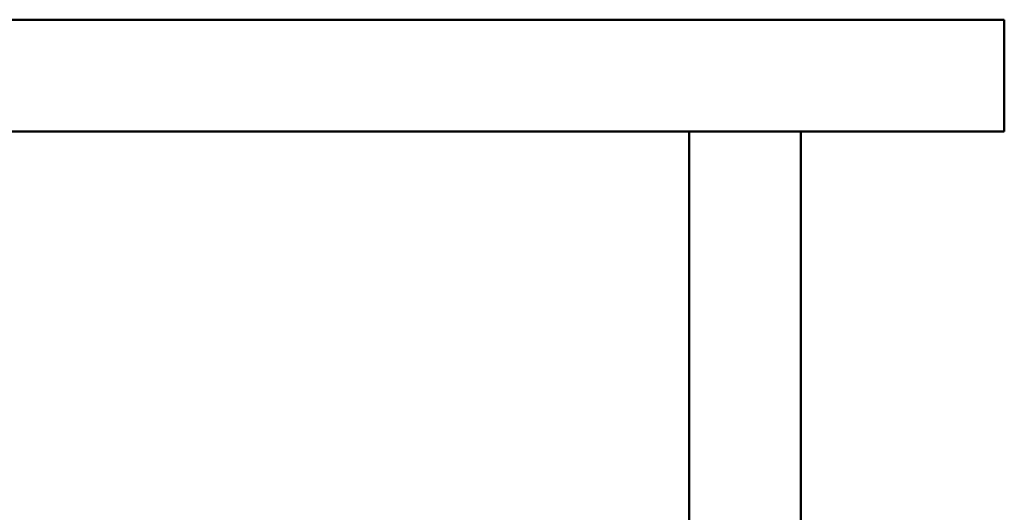
# Model space of a CAD drawing. Units: inches. Extents: x 64 to 1167, y 117 to 939.
# Tile 11 of 56: x 210 to 246, y 620 to 637. Entities that reach past the tile are written whole.
import ezdxf

# ---------------------------------------------------------------- set-up
doc = ezdxf.new("R2010")
doc.units = ezdxf.units.IN
doc.header["$MEASUREMENT"] = 0
doc.layers.add('A-WALL', color=7, linetype='Continuous', lineweight=50)

msp = doc.modelspace()

# ---------------------------------------------------------------- linework, layer by layer
at = {"layer": 'A-WALL'}
for p, q in [((245.609, 637.2), (131.107, 637.2)), ((245.609, 637.2), (245.609, 633.2)), ((245.609, 633.2), (131.107, 633.2)), ((234.326, 633.2), (234.326, 585.2)), ((238.326, 633.2), (238.326, 585.2))]:
    msp.add_line(p, q, dxfattribs=at)

doc.saveas('drawing.dxf')
